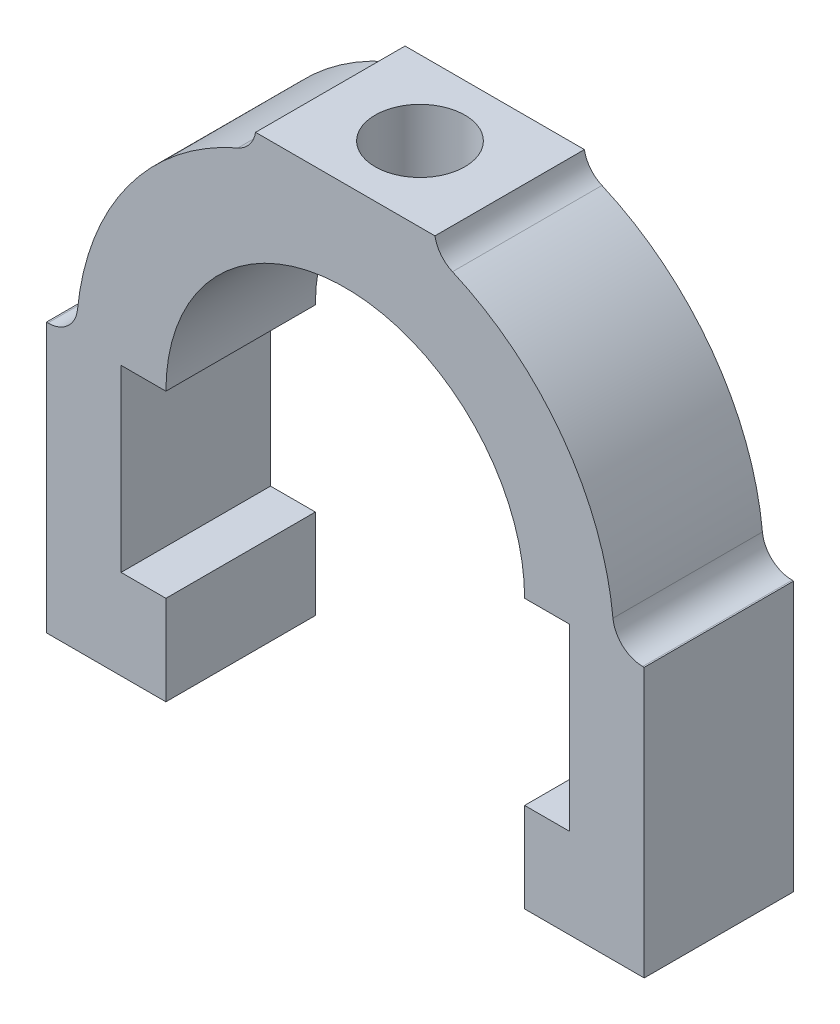
ISO-10303-21;
HEADER;
FILE_DESCRIPTION(('STEP AP214'),'2;1');
FILE_NAME('part.step','',(''),(''),'','','');
FILE_SCHEMA(('AUTOMOTIVE_DESIGN { 1 0 10303 214 1 1 1 1 }'));
ENDSEC;
DATA;
#1=APPLICATION_CONTEXT('core data for automotive mechanical design processes');
#2=APPLICATION_PROTOCOL_DEFINITION('international standard','automotive_design',2000,#1);
#3=PRODUCT_CONTEXT('',#1,'mechanical');
#4=PRODUCT('Part','Part','',(#3));
#5=PRODUCT_RELATED_PRODUCT_CATEGORY('part','',(#4));
#6=PRODUCT_DEFINITION_FORMATION('','',#4);
#7=PRODUCT_DEFINITION_CONTEXT('part definition',#1,'design');
#8=PRODUCT_DEFINITION('design','',#6,#7);
#9=PRODUCT_DEFINITION_SHAPE('','',#8);
#10=(LENGTH_UNIT() NAMED_UNIT(*) SI_UNIT(.MILLI.,.METRE.));
#11=(NAMED_UNIT(*) PLANE_ANGLE_UNIT() SI_UNIT($,.RADIAN.));
#12=(NAMED_UNIT(*) SI_UNIT($,.STERADIAN.) SOLID_ANGLE_UNIT());
#13=UNCERTAINTY_MEASURE_WITH_UNIT(LENGTH_MEASURE(1.E-05),#10,'distance_accuracy_value','');
#14=(GEOMETRIC_REPRESENTATION_CONTEXT(3) GLOBAL_UNCERTAINTY_ASSIGNED_CONTEXT((#13)) GLOBAL_UNIT_ASSIGNED_CONTEXT((#10,
#11,#12)) REPRESENTATION_CONTEXT('',''));
#15=CARTESIAN_POINT('',(0.,0.,0.));
#16=DIRECTION('',(0.,0.,1.));
#17=DIRECTION('',(1.,0.,0.));
#18=AXIS2_PLACEMENT_3D('',#15,#16,#17);
#19=CARTESIAN_POINT('',(0.,36.,-20.));
#20=DIRECTION('',(0.,0.,1.));
#21=DIRECTION('',(1.,0.,0.));
#22=AXIS2_PLACEMENT_3D('',#19,#20,#21);
#23=CYLINDRICAL_SURFACE('',#22,36.);
#24=CARTESIAN_POINT('',(0.,36.,-20.));
#25=DIRECTION('',(0.,0.,1.));
#26=DIRECTION('',(1.,0.,0.));
#27=AXIS2_PLACEMENT_3D('',#24,#25,#26);
#28=CIRCLE('',#27,36.);
#29=CARTESIAN_POINT('',(35.8195477358383,39.6,-20.));
#30=VERTEX_POINT('',#29);
#31=CARTESIAN_POINT('',(14.3465927559282,69.0178024146906,-20.));
#32=VERTEX_POINT('',#31);
#33=EDGE_CURVE('E302',#30,#32,#28,.T.);
#34=ORIENTED_EDGE('',*,*,#33,.T.);
#35=DIRECTION('',(0.,0.,1.));
#36=VECTOR('',#35,1.);
#37=CARTESIAN_POINT('',(14.3465927559282,69.0178024146906,-20.));
#38=LINE('',#37,#36);
#39=CARTESIAN_POINT('',(14.3465927559282,69.0178024146906,0.));
#40=VERTEX_POINT('',#39);
#41=EDGE_CURVE('E377',#32,#40,#38,.T.);
#42=ORIENTED_EDGE('',*,*,#41,.T.);
#43=CARTESIAN_POINT('',(0.,36.,0.));
#44=DIRECTION('',(0.,0.,1.));
#45=DIRECTION('',(1.,0.,0.));
#46=AXIS2_PLACEMENT_3D('',#43,#44,#45);
#47=CIRCLE('',#46,36.);
#48=CARTESIAN_POINT('',(35.8195477358383,39.6,0.));
#49=VERTEX_POINT('',#48);
#50=EDGE_CURVE('E330',#49,#40,#47,.T.);
#51=ORIENTED_EDGE('',*,*,#50,.F.);
#52=DIRECTION('',(0.,0.,1.));
#53=VECTOR('',#52,1.);
#54=CARTESIAN_POINT('',(35.8195477358383,39.6,-20.));
#55=LINE('',#54,#53);
#56=EDGE_CURVE('E361',#49,#30,#55,.F.);
#57=ORIENTED_EDGE('',*,*,#56,.T.);
#58=EDGE_LOOP('',(#34,#42,#51,#57));
#59=FACE_BOUND('',#58,.T.);
#60=ADVANCED_FACE('F58',(#59),#23,.T.);
#61=CARTESIAN_POINT('',(-14.3465927559282,69.0178024146906,0.));
#62=VERTEX_POINT('',#61);
#63=CARTESIAN_POINT('',(-35.8195477358383,39.6,0.));
#64=VERTEX_POINT('',#63);
#65=EDGE_CURVE('E327',#62,#64,#47,.T.);
#66=ORIENTED_EDGE('',*,*,#65,.F.);
#67=DIRECTION('',(0.,0.,1.));
#68=VECTOR('',#67,1.);
#69=CARTESIAN_POINT('',(-14.3465927559282,69.0178024146906,-20.));
#70=LINE('',#69,#68);
#71=CARTESIAN_POINT('',(-14.3465927559282,69.0178024146906,-20.));
#72=VERTEX_POINT('',#71);
#73=EDGE_CURVE('E84',#62,#72,#70,.F.);
#74=ORIENTED_EDGE('',*,*,#73,.T.);
#75=CARTESIAN_POINT('',(-35.8195477358383,39.6,-20.));
#76=VERTEX_POINT('',#75);
#77=EDGE_CURVE('E211',#72,#76,#28,.T.);
#78=ORIENTED_EDGE('',*,*,#77,.T.);
#79=DIRECTION('',(0.,0.,1.));
#80=VECTOR('',#79,1.);
#81=CARTESIAN_POINT('',(-35.8195477358383,39.6,-20.));
#82=LINE('',#81,#80);
#83=EDGE_CURVE('E367',#76,#64,#82,.T.);
#84=ORIENTED_EDGE('',*,*,#83,.T.);
#85=EDGE_LOOP('',(#66,#74,#78,#84));
#86=FACE_BOUND('',#85,.T.);
#87=ADVANCED_FACE('F462',(#86),#23,.T.);
#88=CARTESIAN_POINT('',(-24.,0.,-20.));
#89=DIRECTION('',(-1.,0.,0.));
#90=DIRECTION('',(0.,0.,1.));
#91=AXIS2_PLACEMENT_3D('',#88,#89,#90);
#92=PLANE('',#91);
#93=DIRECTION('',(0.,-1.,0.));
#94=VECTOR('',#93,1.);
#95=CARTESIAN_POINT('',(-24.,0.,-20.));
#96=LINE('',#95,#94);
#97=CARTESIAN_POINT('',(-24.,12.,-20.));
#98=VERTEX_POINT('',#97);
#99=CARTESIAN_POINT('',(-24.,0.,-20.));
#100=VERTEX_POINT('',#99);
#101=EDGE_CURVE('E314',#98,#100,#96,.T.);
#102=ORIENTED_EDGE('',*,*,#101,.F.);
#103=DIRECTION('',(0.,0.,1.));
#104=VECTOR('',#103,1.);
#105=CARTESIAN_POINT('',(-24.,12.,-178.));
#106=LINE('',#105,#104);
#107=CARTESIAN_POINT('',(-24.,12.,0.));
#108=VERTEX_POINT('',#107);
#109=EDGE_CURVE('E242',#98,#108,#106,.T.);
#110=ORIENTED_EDGE('',*,*,#109,.T.);
#111=DIRECTION('',(0.,-1.,0.));
#112=VECTOR('',#111,1.);
#113=CARTESIAN_POINT('',(-24.,0.,0.));
#114=LINE('',#113,#112);
#115=CARTESIAN_POINT('',(-24.,0.,0.));
#116=VERTEX_POINT('',#115);
#117=EDGE_CURVE('E294',#108,#116,#114,.T.);
#118=ORIENTED_EDGE('',*,*,#117,.T.);
#119=DIRECTION('',(0.,0.,1.));
#120=VECTOR('',#119,1.);
#121=CARTESIAN_POINT('',(-24.,0.,-20.));
#122=LINE('',#121,#120);
#123=EDGE_CURVE('E343',#100,#116,#122,.T.);
#124=ORIENTED_EDGE('',*,*,#123,.F.);
#125=EDGE_LOOP('',(#102,#110,#118,#124));
#126=FACE_BOUND('',#125,.T.);
#127=ADVANCED_FACE('F447',(#126),#92,.F.);
#128=CARTESIAN_POINT('',(0.,0.,-20.));
#129=DIRECTION('',(0.,-1.,0.));
#130=DIRECTION('',(0.,0.,-1.));
#131=AXIS2_PLACEMENT_3D('',#128,#129,#130);
#132=PLANE('',#131);
#133=DIRECTION('',(1.,0.,0.));
#134=VECTOR('',#133,1.);
#135=CARTESIAN_POINT('',(0.,0.,0.));
#136=LINE('',#135,#134);
#137=CARTESIAN_POINT('',(-40.,0.,0.));
#138=VERTEX_POINT('',#137);
#139=EDGE_CURVE('E340',#138,#116,#136,.T.);
#140=ORIENTED_EDGE('',*,*,#139,.F.);
#141=DIRECTION('',(0.,0.,1.));
#142=VECTOR('',#141,1.);
#143=CARTESIAN_POINT('',(-40.,0.,-20.));
#144=LINE('',#143,#142);
#145=CARTESIAN_POINT('',(-40.,0.,-20.));
#146=VERTEX_POINT('',#145);
#147=EDGE_CURVE('E349',#146,#138,#144,.T.);
#148=ORIENTED_EDGE('',*,*,#147,.F.);
#149=DIRECTION('',(1.,0.,0.));
#150=VECTOR('',#149,1.);
#151=CARTESIAN_POINT('',(0.,0.,-20.));
#152=LINE('',#151,#150);
#153=EDGE_CURVE('E315',#146,#100,#152,.T.);
#154=ORIENTED_EDGE('',*,*,#153,.T.);
#155=ORIENTED_EDGE('',*,*,#123,.T.);
#156=EDGE_LOOP('',(#140,#148,#154,#155));
#157=FACE_BOUND('',#156,.T.);
#158=ADVANCED_FACE('F446',(#157),#132,.T.);
#159=CARTESIAN_POINT('',(-40.,0.,-20.));
#160=DIRECTION('',(1.,0.,0.));
#161=DIRECTION('',(0.,0.,-1.));
#162=AXIS2_PLACEMENT_3D('',#159,#160,#161);
#163=PLANE('',#162);
#164=DIRECTION('',(0.,1.,0.));
#165=VECTOR('',#164,1.);
#166=CARTESIAN_POINT('',(-40.,0.,0.));
#167=LINE('',#166,#165);
#168=CARTESIAN_POINT('',(-40.,36.,0.));
#169=VERTEX_POINT('',#168);
#170=EDGE_CURVE('E332',#138,#169,#167,.T.);
#171=ORIENTED_EDGE('',*,*,#170,.T.);
#172=DIRECTION('',(0.,0.,1.));
#173=VECTOR('',#172,1.);
#174=CARTESIAN_POINT('',(-40.,36.,-20.));
#175=LINE('',#174,#173);
#176=CARTESIAN_POINT('',(-40.,36.,-20.));
#177=VERTEX_POINT('',#176);
#178=EDGE_CURVE('E350',#177,#169,#175,.T.);
#179=ORIENTED_EDGE('',*,*,#178,.F.);
#180=DIRECTION('',(0.,1.,0.));
#181=VECTOR('',#180,1.);
#182=CARTESIAN_POINT('',(-40.,0.,-20.));
#183=LINE('',#182,#181);
#184=EDGE_CURVE('E309',#146,#177,#183,.T.);
#185=ORIENTED_EDGE('',*,*,#184,.F.);
#186=ORIENTED_EDGE('',*,*,#147,.T.);
#187=EDGE_LOOP('',(#171,#179,#185,#186));
#188=FACE_BOUND('',#187,.T.);
#189=ADVANCED_FACE('F452',(#188),#163,.F.);
#190=CARTESIAN_POINT('',(0.,36.,-20.));
#191=DIRECTION('',(0.,-1.,0.));
#192=DIRECTION('',(0.,0.,-1.));
#193=AXIS2_PLACEMENT_3D('',#190,#191,#192);
#194=PLANE('',#193);
#195=DIRECTION('',(1.,0.,0.));
#196=VECTOR('',#195,1.);
#197=CARTESIAN_POINT('',(0.,36.,0.));
#198=LINE('',#197,#196);
#199=CARTESIAN_POINT('',(-39.7994974842648,36.,0.));
#200=VERTEX_POINT('',#199);
#201=EDGE_CURVE('E331',#169,#200,#198,.T.);
#202=ORIENTED_EDGE('',*,*,#201,.T.);
#203=DIRECTION('',(0.,0.,1.));
#204=VECTOR('',#203,1.);
#205=CARTESIAN_POINT('',(-39.7994974842648,36.,-20.));
#206=LINE('',#205,#204);
#207=CARTESIAN_POINT('',(-39.7994974842648,36.,-20.));
#208=VERTEX_POINT('',#207);
#209=EDGE_CURVE('E375',#200,#208,#206,.F.);
#210=ORIENTED_EDGE('',*,*,#209,.T.);
#211=DIRECTION('',(1.,0.,0.));
#212=VECTOR('',#211,1.);
#213=CARTESIAN_POINT('',(0.,36.,-20.));
#214=LINE('',#213,#212);
#215=EDGE_CURVE('E310',#177,#208,#214,.T.);
#216=ORIENTED_EDGE('',*,*,#215,.F.);
#217=ORIENTED_EDGE('',*,*,#178,.T.);
#218=EDGE_LOOP('',(#202,#210,#216,#217));
#219=FACE_BOUND('',#218,.T.);
#220=ADVANCED_FACE('F460',(#219),#194,.F.);
#221=CARTESIAN_POINT('',(0.,36.,-20.));
#222=DIRECTION('',(0.,1.,0.));
#223=DIRECTION('',(0.,0.,1.));
#224=AXIS2_PLACEMENT_3D('',#221,#222,#223);
#225=PLANE('',#224);
#226=DIRECTION('',(-1.,0.,0.));
#227=VECTOR('',#226,1.);
#228=CARTESIAN_POINT('',(0.,36.,-20.));
#229=LINE('',#228,#227);
#230=CARTESIAN_POINT('',(40.,36.,-20.));
#231=VERTEX_POINT('',#230);
#232=CARTESIAN_POINT('',(39.7994974842648,36.,-20.));
#233=VERTEX_POINT('',#232);
#234=EDGE_CURVE('E301',#231,#233,#229,.T.);
#235=ORIENTED_EDGE('',*,*,#234,.T.);
#236=DIRECTION('',(0.,0.,-1.));
#237=VECTOR('',#236,1.);
#238=CARTESIAN_POINT('',(39.7994974842648,36.,0.));
#239=LINE('',#238,#237);
#240=CARTESIAN_POINT('',(39.7994974842648,36.,0.));
#241=VERTEX_POINT('',#240);
#242=EDGE_CURVE('E345',#233,#241,#239,.F.);
#243=ORIENTED_EDGE('',*,*,#242,.T.);
#244=DIRECTION('',(-1.,0.,0.));
#245=VECTOR('',#244,1.);
#246=CARTESIAN_POINT('',(0.,36.,0.));
#247=LINE('',#246,#245);
#248=CARTESIAN_POINT('',(40.,36.,0.));
#249=VERTEX_POINT('',#248);
#250=EDGE_CURVE('E322',#249,#241,#247,.T.);
#251=ORIENTED_EDGE('',*,*,#250,.F.);
#252=DIRECTION('',(0.,0.,1.));
#253=VECTOR('',#252,1.);
#254=CARTESIAN_POINT('',(40.,36.,-20.));
#255=LINE('',#254,#253);
#256=EDGE_CURVE('E351',#231,#249,#255,.T.);
#257=ORIENTED_EDGE('',*,*,#256,.F.);
#258=EDGE_LOOP('',(#235,#243,#251,#257));
#259=FACE_BOUND('',#258,.T.);
#260=ADVANCED_FACE('F402',(#259),#225,.T.);
#261=CARTESIAN_POINT('',(40.,0.,-20.));
#262=DIRECTION('',(1.,0.,0.));
#263=DIRECTION('',(0.,0.,-1.));
#264=AXIS2_PLACEMENT_3D('',#261,#262,#263);
#265=PLANE('',#264);
#266=DIRECTION('',(0.,1.,0.));
#267=VECTOR('',#266,1.);
#268=CARTESIAN_POINT('',(40.,0.,0.));
#269=LINE('',#268,#267);
#270=CARTESIAN_POINT('',(40.,0.,0.));
#271=VERTEX_POINT('',#270);
#272=EDGE_CURVE('E321',#271,#249,#269,.T.);
#273=ORIENTED_EDGE('',*,*,#272,.F.);
#274=DIRECTION('',(0.,0.,1.));
#275=VECTOR('',#274,1.);
#276=CARTESIAN_POINT('',(40.,0.,-20.));
#277=LINE('',#276,#275);
#278=CARTESIAN_POINT('',(40.,0.,-20.));
#279=VERTEX_POINT('',#278);
#280=EDGE_CURVE('E353',#279,#271,#277,.T.);
#281=ORIENTED_EDGE('',*,*,#280,.F.);
#282=DIRECTION('',(0.,1.,0.));
#283=VECTOR('',#282,1.);
#284=CARTESIAN_POINT('',(40.,0.,-20.));
#285=LINE('',#284,#283);
#286=EDGE_CURVE('E296',#279,#231,#285,.T.);
#287=ORIENTED_EDGE('',*,*,#286,.T.);
#288=ORIENTED_EDGE('',*,*,#256,.T.);
#289=EDGE_LOOP('',(#273,#281,#287,#288));
#290=FACE_BOUND('',#289,.T.);
#291=ADVANCED_FACE('F403',(#290),#265,.T.);
#292=CARTESIAN_POINT('',(0.,0.,-20.));
#293=DIRECTION('',(0.,-1.,0.));
#294=DIRECTION('',(0.,0.,-1.));
#295=AXIS2_PLACEMENT_3D('',#292,#293,#294);
#296=PLANE('',#295);
#297=DIRECTION('',(1.,0.,0.));
#298=VECTOR('',#297,1.);
#299=CARTESIAN_POINT('',(0.,0.,0.));
#300=LINE('',#299,#298);
#301=CARTESIAN_POINT('',(24.,0.,0.));
#302=VERTEX_POINT('',#301);
#303=EDGE_CURVE('E316',#302,#271,#300,.T.);
#304=ORIENTED_EDGE('',*,*,#303,.F.);
#305=DIRECTION('',(0.,0.,1.));
#306=VECTOR('',#305,1.);
#307=CARTESIAN_POINT('',(24.,0.,-20.));
#308=LINE('',#307,#306);
#309=CARTESIAN_POINT('',(24.,0.,-20.));
#310=VERTEX_POINT('',#309);
#311=EDGE_CURVE('E358',#310,#302,#308,.T.);
#312=ORIENTED_EDGE('',*,*,#311,.F.);
#313=DIRECTION('',(1.,0.,0.));
#314=VECTOR('',#313,1.);
#315=CARTESIAN_POINT('',(0.,0.,-20.));
#316=LINE('',#315,#314);
#317=EDGE_CURVE('E295',#310,#279,#316,.T.);
#318=ORIENTED_EDGE('',*,*,#317,.T.);
#319=ORIENTED_EDGE('',*,*,#280,.T.);
#320=EDGE_LOOP('',(#304,#312,#318,#319));
#321=FACE_BOUND('',#320,.T.);
#322=ADVANCED_FACE('F413',(#321),#296,.T.);
#323=CARTESIAN_POINT('',(24.,0.,-20.));
#324=DIRECTION('',(-1.,0.,0.));
#325=DIRECTION('',(0.,0.,1.));
#326=AXIS2_PLACEMENT_3D('',#323,#324,#325);
#327=PLANE('',#326);
#328=DIRECTION('',(0.,0.,1.));
#329=VECTOR('',#328,1.);
#330=CARTESIAN_POINT('',(24.,12.,-178.));
#331=LINE('',#330,#329);
#332=CARTESIAN_POINT('',(24.,12.,-20.));
#333=VERTEX_POINT('',#332);
#334=CARTESIAN_POINT('',(24.,12.,0.));
#335=VERTEX_POINT('',#334);
#336=EDGE_CURVE('E248',#333,#335,#331,.T.);
#337=ORIENTED_EDGE('',*,*,#336,.F.);
#338=DIRECTION('',(0.,-1.,0.));
#339=VECTOR('',#338,1.);
#340=CARTESIAN_POINT('',(24.,0.,-20.));
#341=LINE('',#340,#339);
#342=EDGE_CURVE('E292',#333,#310,#341,.T.);
#343=ORIENTED_EDGE('',*,*,#342,.T.);
#344=ORIENTED_EDGE('',*,*,#311,.T.);
#345=DIRECTION('',(0.,-1.,0.));
#346=VECTOR('',#345,1.);
#347=CARTESIAN_POINT('',(24.,0.,0.));
#348=LINE('',#347,#346);
#349=EDGE_CURVE('E293',#335,#302,#348,.T.);
#350=ORIENTED_EDGE('',*,*,#349,.F.);
#351=EDGE_LOOP('',(#337,#343,#344,#350));
#352=FACE_BOUND('',#351,.T.);
#353=ADVANCED_FACE('F411',(#352),#327,.T.);
#354=CARTESIAN_POINT('',(0.,0.,-20.));
#355=DIRECTION('',(0.,0.,1.));
#356=DIRECTION('',(1.,0.,0.));
#357=AXIS2_PLACEMENT_3D('',#354,#355,#356);
#358=PLANE('',#357);
#359=DIRECTION('',(0.,1.,0.));
#360=VECTOR('',#359,1.);
#361=CARTESIAN_POINT('',(30.,0.,-20.));
#362=LINE('',#361,#360);
#363=CARTESIAN_POINT('',(30.,12.,-20.));
#364=VERTEX_POINT('',#363);
#365=CARTESIAN_POINT('',(30.,36.,-20.));
#366=VERTEX_POINT('',#365);
#367=EDGE_CURVE('E282',#364,#366,#362,.T.);
#368=ORIENTED_EDGE('',*,*,#367,.T.);
#369=DIRECTION('',(-1.,0.,0.));
#370=VECTOR('',#369,1.);
#371=CARTESIAN_POINT('',(0.,36.,-20.));
#372=LINE('',#371,#370);
#373=CARTESIAN_POINT('',(24.,36.,-20.));
#374=VERTEX_POINT('',#373);
#375=EDGE_CURVE('E272',#366,#374,#372,.T.);
#376=ORIENTED_EDGE('',*,*,#375,.T.);
#377=CARTESIAN_POINT('',(0.,36.,-20.));
#378=DIRECTION('',(0.,0.,1.));
#379=DIRECTION('',(1.,0.,0.));
#380=AXIS2_PLACEMENT_3D('',#377,#378,#379);
#381=CIRCLE('',#380,24.);
#382=CARTESIAN_POINT('',(-24.,36.,-20.));
#383=VERTEX_POINT('',#382);
#384=EDGE_CURVE('E290',#374,#383,#381,.T.);
#385=ORIENTED_EDGE('',*,*,#384,.T.);
#386=DIRECTION('',(-1.,0.,0.));
#387=VECTOR('',#386,1.);
#388=CARTESIAN_POINT('',(0.,36.,-20.));
#389=LINE('',#388,#387);
#390=CARTESIAN_POINT('',(-30.,36.,-20.));
#391=VERTEX_POINT('',#390);
#392=EDGE_CURVE('E255',#383,#391,#389,.T.);
#393=ORIENTED_EDGE('',*,*,#392,.T.);
#394=DIRECTION('',(0.,-1.,0.));
#395=VECTOR('',#394,1.);
#396=CARTESIAN_POINT('',(-30.,0.,-20.));
#397=LINE('',#396,#395);
#398=CARTESIAN_POINT('',(-30.,12.,-20.));
#399=VERTEX_POINT('',#398);
#400=EDGE_CURVE('E274',#391,#399,#397,.T.);
#401=ORIENTED_EDGE('',*,*,#400,.T.);
#402=DIRECTION('',(1.,0.,0.));
#403=VECTOR('',#402,1.);
#404=CARTESIAN_POINT('',(0.,12.,-20.));
#405=LINE('',#404,#403);
#406=EDGE_CURVE('E276',#399,#98,#405,.T.);
#407=ORIENTED_EDGE('',*,*,#406,.T.);
#408=ORIENTED_EDGE('',*,*,#101,.T.);
#409=ORIENTED_EDGE('',*,*,#153,.F.);
#410=ORIENTED_EDGE('',*,*,#184,.T.);
#411=ORIENTED_EDGE('',*,*,#215,.T.);
#412=CARTESIAN_POINT('',(-39.7994974842648,40.,-20.));
#413=DIRECTION('',(0.,0.,1.));
#414=DIRECTION('',(1.,0.,0.));
#415=AXIS2_PLACEMENT_3D('',#412,#413,#414);
#416=CIRCLE('',#415,4.);
#417=EDGE_CURVE('E376',#208,#76,#416,.T.);
#418=ORIENTED_EDGE('',*,*,#417,.T.);
#419=ORIENTED_EDGE('',*,*,#77,.F.);
#420=CARTESIAN_POINT('',(-15.940658617698,72.686447127434,-20.));
#421=DIRECTION('',(0.,0.,1.));
#422=DIRECTION('',(1.,0.,0.));
#423=AXIS2_PLACEMENT_3D('',#420,#421,#422);
#424=CIRCLE('',#423,4.);
#425=CARTESIAN_POINT('',(-12.,72.,-20.));
#426=VERTEX_POINT('',#425);
#427=EDGE_CURVE('E12',#72,#426,#424,.T.);
#428=ORIENTED_EDGE('',*,*,#427,.T.);
#429=DIRECTION('',(1.,0.,0.));
#430=VECTOR('',#429,1.);
#431=CARTESIAN_POINT('',(0.,72.,-20.));
#432=LINE('',#431,#430);
#433=CARTESIAN_POINT('',(12.,72.,-20.));
#434=VERTEX_POINT('',#433);
#435=EDGE_CURVE('E209',#426,#434,#432,.T.);
#436=ORIENTED_EDGE('',*,*,#435,.T.);
#437=CARTESIAN_POINT('',(15.940658617698,72.686447127434,-20.));
#438=DIRECTION('',(0.,0.,1.));
#439=DIRECTION('',(1.,0.,0.));
#440=AXIS2_PLACEMENT_3D('',#437,#438,#439);
#441=CIRCLE('',#440,4.);
#442=EDGE_CURVE('E384',#434,#32,#441,.T.);
#443=ORIENTED_EDGE('',*,*,#442,.T.);
#444=ORIENTED_EDGE('',*,*,#33,.F.);
#445=CARTESIAN_POINT('',(39.7994974842648,40.,-20.));
#446=DIRECTION('',(0.,0.,1.));
#447=DIRECTION('',(1.,0.,0.));
#448=AXIS2_PLACEMENT_3D('',#445,#446,#447);
#449=CIRCLE('',#448,4.);
#450=EDGE_CURVE('E370',#30,#233,#449,.T.);
#451=ORIENTED_EDGE('',*,*,#450,.T.);
#452=ORIENTED_EDGE('',*,*,#234,.F.);
#453=ORIENTED_EDGE('',*,*,#286,.F.);
#454=ORIENTED_EDGE('',*,*,#317,.F.);
#455=ORIENTED_EDGE('',*,*,#342,.F.);
#456=DIRECTION('',(1.,0.,0.));
#457=VECTOR('',#456,1.);
#458=CARTESIAN_POINT('',(0.,12.,-20.));
#459=LINE('',#458,#457);
#460=EDGE_CURVE('E277',#333,#364,#459,.T.);
#461=ORIENTED_EDGE('',*,*,#460,.T.);
#462=EDGE_LOOP('',(#368,#376,#385,#393,#401,#407,#408,#409,#410,#411,#418,#419,#428,#436,#443,
#444,#451,#452,#453,#454,#455,#461));
#463=FACE_BOUND('',#462,.T.);
#464=ADVANCED_FACE('F206',(#463),#358,.F.);
#465=CARTESIAN_POINT('',(0.,0.,0.));
#466=DIRECTION('',(0.,0.,1.));
#467=DIRECTION('',(1.,0.,0.));
#468=AXIS2_PLACEMENT_3D('',#465,#466,#467);
#469=PLANE('',#468);
#470=DIRECTION('',(-1.,0.,0.));
#471=VECTOR('',#470,1.);
#472=CARTESIAN_POINT('',(30.,36.,0.));
#473=LINE('',#472,#471);
#474=CARTESIAN_POINT('',(30.,36.,0.));
#475=VERTEX_POINT('',#474);
#476=CARTESIAN_POINT('',(24.,36.,0.));
#477=VERTEX_POINT('',#476);
#478=EDGE_CURVE('E250',#475,#477,#473,.T.);
#479=ORIENTED_EDGE('',*,*,#478,.F.);
#480=DIRECTION('',(0.,1.,0.));
#481=VECTOR('',#480,1.);
#482=CARTESIAN_POINT('',(30.,12.,0.));
#483=LINE('',#482,#481);
#484=CARTESIAN_POINT('',(30.,12.,0.));
#485=VERTEX_POINT('',#484);
#486=EDGE_CURVE('E243',#485,#475,#483,.T.);
#487=ORIENTED_EDGE('',*,*,#486,.F.);
#488=DIRECTION('',(1.,0.,0.));
#489=VECTOR('',#488,1.);
#490=CARTESIAN_POINT('',(24.,12.,0.));
#491=LINE('',#490,#489);
#492=EDGE_CURVE('E239',#335,#485,#491,.T.);
#493=ORIENTED_EDGE('',*,*,#492,.F.);
#494=ORIENTED_EDGE('',*,*,#349,.T.);
#495=ORIENTED_EDGE('',*,*,#303,.T.);
#496=ORIENTED_EDGE('',*,*,#272,.T.);
#497=ORIENTED_EDGE('',*,*,#250,.T.);
#498=CARTESIAN_POINT('',(39.7994974842648,40.,0.));
#499=DIRECTION('',(0.,0.,1.));
#500=DIRECTION('',(1.,0.,0.));
#501=AXIS2_PLACEMENT_3D('',#498,#499,#500);
#502=CIRCLE('',#501,4.);
#503=EDGE_CURVE('E362',#241,#49,#502,.F.);
#504=ORIENTED_EDGE('',*,*,#503,.T.);
#505=ORIENTED_EDGE('',*,*,#50,.T.);
#506=CARTESIAN_POINT('',(15.940658617698,72.686447127434,0.));
#507=DIRECTION('',(0.,0.,1.));
#508=DIRECTION('',(1.,0.,0.));
#509=AXIS2_PLACEMENT_3D('',#506,#507,#508);
#510=CIRCLE('',#509,4.);
#511=CARTESIAN_POINT('',(12.,72.,0.));
#512=VERTEX_POINT('',#511);
#513=EDGE_CURVE('E382',#40,#512,#510,.F.);
#514=ORIENTED_EDGE('',*,*,#513,.T.);
#515=DIRECTION('',(1.,0.,0.));
#516=VECTOR('',#515,1.);
#517=CARTESIAN_POINT('',(0.,72.,0.));
#518=LINE('',#517,#516);
#519=CARTESIAN_POINT('',(-12.,72.,0.));
#520=VERTEX_POINT('',#519);
#521=EDGE_CURVE('E225',#520,#512,#518,.T.);
#522=ORIENTED_EDGE('',*,*,#521,.F.);
#523=CARTESIAN_POINT('',(-15.940658617698,72.686447127434,0.));
#524=DIRECTION('',(0.,0.,1.));
#525=DIRECTION('',(1.,0.,0.));
#526=AXIS2_PLACEMENT_3D('',#523,#524,#525);
#527=CIRCLE('',#526,4.);
#528=EDGE_CURVE('E67',#520,#62,#527,.F.);
#529=ORIENTED_EDGE('',*,*,#528,.T.);
#530=ORIENTED_EDGE('',*,*,#65,.T.);
#531=CARTESIAN_POINT('',(-39.7994974842648,40.,0.));
#532=DIRECTION('',(0.,0.,1.));
#533=DIRECTION('',(1.,0.,0.));
#534=AXIS2_PLACEMENT_3D('',#531,#532,#533);
#535=CIRCLE('',#534,4.);
#536=EDGE_CURVE('E372',#64,#200,#535,.F.);
#537=ORIENTED_EDGE('',*,*,#536,.T.);
#538=ORIENTED_EDGE('',*,*,#201,.F.);
#539=ORIENTED_EDGE('',*,*,#170,.F.);
#540=ORIENTED_EDGE('',*,*,#139,.T.);
#541=ORIENTED_EDGE('',*,*,#117,.F.);
#542=DIRECTION('',(1.,0.,0.));
#543=VECTOR('',#542,1.);
#544=CARTESIAN_POINT('',(-24.,12.,0.));
#545=LINE('',#544,#543);
#546=CARTESIAN_POINT('',(-30.,12.,0.));
#547=VERTEX_POINT('',#546);
#548=EDGE_CURVE('E263',#547,#108,#545,.T.);
#549=ORIENTED_EDGE('',*,*,#548,.F.);
#550=DIRECTION('',(0.,-1.,0.));
#551=VECTOR('',#550,1.);
#552=CARTESIAN_POINT('',(-30.,12.,0.));
#553=LINE('',#552,#551);
#554=CARTESIAN_POINT('',(-30.,36.,0.));
#555=VERTEX_POINT('',#554);
#556=EDGE_CURVE('E260',#555,#547,#553,.T.);
#557=ORIENTED_EDGE('',*,*,#556,.F.);
#558=DIRECTION('',(-1.,0.,0.));
#559=VECTOR('',#558,1.);
#560=CARTESIAN_POINT('',(-30.,36.,0.));
#561=LINE('',#560,#559);
#562=CARTESIAN_POINT('',(-24.,36.,0.));
#563=VERTEX_POINT('',#562);
#564=EDGE_CURVE('E237',#563,#555,#561,.T.);
#565=ORIENTED_EDGE('',*,*,#564,.F.);
#566=CARTESIAN_POINT('',(0.,36.,0.));
#567=DIRECTION('',(0.,0.,1.));
#568=DIRECTION('',(1.,0.,0.));
#569=AXIS2_PLACEMENT_3D('',#566,#567,#568);
#570=CIRCLE('',#569,24.);
#571=EDGE_CURVE('E281',#477,#563,#570,.T.);
#572=ORIENTED_EDGE('',*,*,#571,.F.);
#573=EDGE_LOOP('',(#479,#487,#493,#494,#495,#496,#497,#504,#505,#514,#522,#529,#530,#537,#538,
#539,#540,#541,#549,#557,#565,#572));
#574=FACE_BOUND('',#573,.T.);
#575=ADVANCED_FACE('F395',(#574),#469,.T.);
#576=CARTESIAN_POINT('',(39.7994974842648,40.,-20.));
#577=DIRECTION('',(0.,0.,1.));
#578=DIRECTION('',(1.,0.,0.));
#579=AXIS2_PLACEMENT_3D('',#576,#577,#578);
#580=CYLINDRICAL_SURFACE('',#579,4.);
#581=ORIENTED_EDGE('',*,*,#450,.F.);
#582=ORIENTED_EDGE('',*,*,#56,.F.);
#583=ORIENTED_EDGE('',*,*,#503,.F.);
#584=ORIENTED_EDGE('',*,*,#242,.F.);
#585=EDGE_LOOP('',(#581,#582,#583,#584));
#586=FACE_BOUND('',#585,.T.);
#587=ADVANCED_FACE('F399',(#586),#580,.F.);
#588=CARTESIAN_POINT('',(-39.7994974842648,40.,-20.));
#589=DIRECTION('',(0.,0.,1.));
#590=DIRECTION('',(1.,0.,0.));
#591=AXIS2_PLACEMENT_3D('',#588,#589,#590);
#592=CYLINDRICAL_SURFACE('',#591,4.);
#593=ORIENTED_EDGE('',*,*,#417,.F.);
#594=ORIENTED_EDGE('',*,*,#209,.F.);
#595=ORIENTED_EDGE('',*,*,#536,.F.);
#596=ORIENTED_EDGE('',*,*,#83,.F.);
#597=EDGE_LOOP('',(#593,#594,#595,#596));
#598=FACE_BOUND('',#597,.T.);
#599=ADVANCED_FACE('F465',(#598),#592,.F.);
#600=CARTESIAN_POINT('',(0.,36.,-31.));
#601=DIRECTION('',(0.,0.,1.));
#602=DIRECTION('',(1.,0.,0.));
#603=AXIS2_PLACEMENT_3D('',#600,#601,#602);
#604=CYLINDRICAL_SURFACE('',#603,24.);
#605=CARTESIAN_POINT('',(0.,60.,-4.));
#606=CARTESIAN_POINT('',(0.165805387403802,60.0000029962766,-3.99999505102641));
#607=CARTESIAN_POINT('',(0.331556618095783,59.9982792337243,-4.00687387489243));
#608=CARTESIAN_POINT('',(0.661898341499742,59.9914389070726,-4.03431986201637));
#609=CARTESIAN_POINT('',(0.826488699612241,59.9863219558732,-4.05488858704015));
#610=CARTESIAN_POINT('',(1.15331468289425,59.9728312747808,-4.10955571939549));
#611=CARTESIAN_POINT('',(1.31554956136034,59.964456534561,-4.14365832400845));
#612=CARTESIAN_POINT('',(1.63652999353389,59.9446785682942,-4.22512392789649));
#613=CARTESIAN_POINT('',(1.7952742379173,59.9332742261501,-4.27249181441513));
#614=CARTESIAN_POINT('',(2.10785890827135,59.9077704080524,-4.38001719827038));
#615=CARTESIAN_POINT('',(2.26170674963502,59.8936752583917,-4.44015418258226));
#616=CARTESIAN_POINT('',(2.56378623821258,59.8631527081916,-4.57282541021577));
#617=CARTESIAN_POINT('',(2.71201578712804,59.8467244469549,-4.64536423066248));
#618=CARTESIAN_POINT('',(3.00177661033544,59.8119848981805,-4.80226274512907));
#619=CARTESIAN_POINT('',(3.1433102969363,59.7936742964516,-4.88661813795178));
#620=CARTESIAN_POINT('',(3.41888526654491,59.7556431475739,-5.06661176459039));
#621=CARTESIAN_POINT('',(3.5529237053449,59.7359220715781,-5.1622542392442));
#622=CARTESIAN_POINT('',(3.81496434602383,59.6952304700178,-5.36598591724915));
#623=CARTESIAN_POINT('',(3.94281308913214,59.674243775966,-5.47426931255561));
#624=CARTESIAN_POINT('',(4.18902736841679,59.6319204183454,-5.70115303311099));
#625=CARTESIAN_POINT('',(4.30738936846955,59.6105836278175,-5.8197571713109));
#626=CARTESIAN_POINT('',(4.53377489524013,59.568159620478,-6.06643888329868));
#627=CARTESIAN_POINT('',(4.64180103185486,59.5470723418473,-6.19451405100954));
#628=CARTESIAN_POINT('',(4.84686316299839,59.5057198367545,-6.45938141653677));
#629=CARTESIAN_POINT('',(4.94389508557169,59.4854549166434,-6.59617681496597));
#630=CARTESIAN_POINT('',(5.12757579334232,59.4460427828086,-6.87960061394558));
#631=CARTESIAN_POINT('',(5.21405329073272,59.4269160793509,-7.02634297896338));
#632=CARTESIAN_POINT('',(5.37434099239073,59.3906650895731,-7.32689631114159));
#633=CARTESIAN_POINT('',(5.4481464054103,59.3735415614194,-7.48070992415988));
#634=CARTESIAN_POINT('',(5.5824381696205,59.3418328254504,-7.79422880998301));
#635=CARTESIAN_POINT('',(5.64293112700069,59.3272463593972,-7.95393111442795));
#636=CARTESIAN_POINT('',(5.75016256060697,59.301043510543,-8.27812298906709));
#637=CARTESIAN_POINT('',(5.79689611131117,59.2894281915327,-8.4426142504887));
#638=CARTESIAN_POINT('',(5.91415157316671,59.2600431044562,-8.93482169258661));
#639=CARTESIAN_POINT('',(5.96458986092324,59.2470332112981,-9.26798361707615));
#640=CARTESIAN_POINT('',(5.99795848349603,59.23842608856,-9.77014845136033));
#641=CARTESIAN_POINT('',(6.00202663613951,59.2373766993858,-9.93800547716951));
#642=CARTESIAN_POINT('',(5.99610970800768,59.2389046091482,-10.2734756491558));
#643=CARTESIAN_POINT('',(5.98612448822742,59.2414819439575,-10.4410887929042));
#644=CARTESIAN_POINT('',(5.93594713474591,59.2543754061852,-10.9334757617709));
#645=CARTESIAN_POINT('',(5.87607363848321,59.2697164452628,-11.2563322349699));
#646=CARTESIAN_POINT('',(5.70489646981085,59.3122664593645,-11.8870944582585));
#647=CARTESIAN_POINT('',(5.59358913348967,59.3394762798586,-12.1949991415238));
#648=CARTESIAN_POINT('',(5.32155798729425,59.4030050803747,-12.7909383990231));
#649=CARTESIAN_POINT('',(5.16034668919655,59.4394132393811,-13.0787410216454));
#650=CARTESIAN_POINT('',(4.79342508379137,59.5171882932266,-13.623678505182));
#651=CARTESIAN_POINT('',(4.58770698972655,59.5585560552156,-13.8808079874003));
#652=CARTESIAN_POINT('',(4.13065370439076,59.6430352608536,-14.3648134392708));
#653=CARTESIAN_POINT('',(3.8781850342093,59.6861627896442,-14.5906176860606));
#654=CARTESIAN_POINT('',(3.33844766846889,59.7682386126258,-14.9968852440488));
#655=CARTESIAN_POINT('',(3.05117791031428,59.8071867791381,-15.1773471702746));
#656=CARTESIAN_POINT('',(2.44846355524484,59.8767092866155,-15.4882022714257));
#657=CARTESIAN_POINT('',(2.13292557335861,59.9072544059235,-15.6184213427058));
#658=CARTESIAN_POINT('',(1.48350403204752,59.9563166788424,-15.8236692411467));
#659=CARTESIAN_POINT('',(1.14962399502517,59.9748361331613,-15.8987086254555));
#660=CARTESIAN_POINT('',(0.482159883096527,59.9974199712544,-15.9898302624469));
#661=CARTESIAN_POINT('',(0.148786885522348,60.0018421411353,-16.0073721225199));
#662=CARTESIAN_POINT('',(-0.516131504775042,59.9967521917739,-15.987003973561));
#663=CARTESIAN_POINT('',(-0.847677059317268,59.987241326857,-15.94909895615));
#664=CARTESIAN_POINT('',(-1.4944570546744,59.9555832478693,-15.8201164380113));
#665=CARTESIAN_POINT('',(-1.80986040015949,59.9336253776701,-15.7298352125968));
#666=CARTESIAN_POINT('',(-2.42102924553322,59.8795482551267,-15.4995713973546));
#667=CARTESIAN_POINT('',(-2.71679275860286,59.8474279766146,-15.3595837881582));
#668=CARTESIAN_POINT('',(-3.28609225023473,59.775732355911,-15.0310564967388));
#669=CARTESIAN_POINT('',(-3.55914068563651,59.7360348408855,-14.8416993592124));
#670=CARTESIAN_POINT('',(-4.07010753646662,59.6537802212633,-14.4208365553548));
#671=CARTESIAN_POINT('',(-4.30801987625634,59.6112226239559,-14.1893236149746));
#672=CARTESIAN_POINT('',(-4.74795813275242,59.5267588379479,-13.6840067323829));
#673=CARTESIAN_POINT('',(-4.94895984477464,59.4848942795269,-13.4093042078171));
#674=CARTESIAN_POINT('',(-5.30205866107054,59.4077130231476,-12.8290144447531));
#675=CARTESIAN_POINT('',(-5.45415793615243,59.3723960345683,-12.5234285779765));
#676=CARTESIAN_POINT('',(-5.6416087071287,59.3275859445682,-12.0496398809846));
#677=CARTESIAN_POINT('',(-5.69722158138527,59.3140336618751,-11.8895567217037));
#678=CARTESIAN_POINT('',(-5.79475769208554,59.2899834650234,-11.5650651703049));
#679=CARTESIAN_POINT('',(-5.83668611505733,59.2794843938355,-11.4006584424464));
#680=CARTESIAN_POINT('',(-5.9064899745362,59.2618715740422,-11.0687170513407));
#681=CARTESIAN_POINT('',(-5.93436517338602,59.2547578826878,-10.901182335245));
#682=CARTESIAN_POINT('',(-5.97582085063046,59.2441396190328,-10.5642421336349));
#683=CARTESIAN_POINT('',(-5.98940200008078,59.2406348773048,-10.3948367363199));
#684=CARTESIAN_POINT('',(-6.00196347285349,59.2373938489065,-10.060331055056));
#685=CARTESIAN_POINT('',(-6.0013522054121,59.2375521518778,-9.89524696865287));
#686=CARTESIAN_POINT('',(-5.98653576306369,59.2413736324535,-9.56573349984315));
#687=CARTESIAN_POINT('',(-5.97233089751311,59.2450367302975,-9.401304102623));
#688=CARTESIAN_POINT('',(-5.93044575509701,59.2557579721328,-9.07425896558782));
#689=CARTESIAN_POINT('',(-5.90276341290372,59.2628166364686,-8.91164350765425));
#690=CARTESIAN_POINT('',(-5.83416667908453,59.2801148571724,-8.58946233314158));
#691=CARTESIAN_POINT('',(-5.79325695086328,59.2903532924404,-8.42989556269428));
#692=CARTESIAN_POINT('',(-5.69880203716712,59.3136441790929,-8.11574761367387));
#693=CARTESIAN_POINT('',(-5.64532943643257,59.3266804293978,-7.96114338738971));
#694=CARTESIAN_POINT('',(-5.52605852883571,59.3552228194459,-7.65706577641293));
#695=CARTESIAN_POINT('',(-5.46026449802037,59.3707281020539,-7.50759063294574));
#696=CARTESIAN_POINT('',(-5.31678835542035,59.4037855982137,-7.21461325501314));
#697=CARTESIAN_POINT('',(-5.23910089912543,59.4213387311534,-7.07111374285786));
#698=CARTESIAN_POINT('',(-5.07243073970643,59.4579990976357,-6.79110854339098));
#699=CARTESIAN_POINT('',(-4.98345174049215,59.4771058208267,-6.65460058319193));
#700=CARTESIAN_POINT('',(-4.7922729032838,59.5168854335111,-6.38585732091633));
#701=CARTESIAN_POINT('',(-4.68978556121475,59.5375863850894,-6.25383061677941));
#702=CARTESIAN_POINT('',(-4.4742434518464,59.579507882839,-5.99887487156699));
#703=CARTESIAN_POINT('',(-4.36119228671727,59.6007282500856,-5.87594275475177));
#704=CARTESIAN_POINT('',(-4.12516419546942,59.6431258862839,-5.63985111466564));
#705=CARTESIAN_POINT('',(-4.0021814457299,59.6643031223737,-5.52669740687929));
#706=CARTESIAN_POINT('',(-3.74719176501411,59.7060168559164,-5.31103132209644));
#707=CARTESIAN_POINT('',(-3.61518813420472,59.7265535837286,-5.2085150877252));
#708=CARTESIAN_POINT('',(-3.34044186706076,59.7668061369628,-5.0129768060556));
#709=CARTESIAN_POINT('',(-3.19754553860501,59.7864996932668,-4.92016593894123));
#710=CARTESIAN_POINT('',(-2.90425652857033,59.824087485808,-4.74697329866601));
#711=CARTESIAN_POINT('',(-2.75386663022821,59.8419823827553,-4.66658695566752));
#712=CARTESIAN_POINT('',(-2.44663692885418,59.8754647710401,-4.51885051284106));
#713=CARTESIAN_POINT('',(-2.28979994155171,59.8910532562916,-4.45149479378778));
#714=CARTESIAN_POINT('',(-1.97079001830644,59.9194829588902,-4.3303336445071));
#715=CARTESIAN_POINT('',(-1.80861789148404,59.9323245906257,-4.27652617018404));
#716=CARTESIAN_POINT('',(-1.3777763047293,59.9619049568243,-4.15376714609566));
#717=CARTESIAN_POINT('',(-1.1055914726577,59.9761014751911,-4.09620462215925));
#718=CARTESIAN_POINT('',(-0.55555350244454,59.9951461360495,-4.01932663186095));
#719=CARTESIAN_POINT('',(-0.277700792219541,59.9999949816564,-4.00000828883734));
#720=CARTESIAN_POINT('',(0.,60.,-4.));
#721=B_SPLINE_CURVE_WITH_KNOTS('',3,(#605,#606,#607,#608,#609,#610,#611,#612,#613,#614,#615,
#616,#617,#618,#619,#620,#621,#622,#623,#624,#625,#626,#627,#628,#629,#630,#631,#632,#633,#634,
#635,#636,#637,#638,#639,#640,#641,#642,#643,#644,#645,#646,#647,#648,#649,#650,#651,#652,#653,
#654,#655,#656,#657,#658,#659,#660,#661,#662,#663,#664,#665,#666,#667,#668,#669,#670,#671,#672,
#673,#674,#675,#676,#677,#678,#679,#680,#681,#682,#683,#684,#685,#686,#687,#688,#689,#690,#691,
#692,#693,#694,#695,#696,#697,#698,#699,#700,#701,#702,#703,#704,#705,#706,#707,#708,#709,#710,
#711,#712,#713,#714,#715,#716,#717,#718,#719,#720),.UNSPECIFIED.,.T.,.F.,(4,2,2,2,2,2,2,2,2,2,2,
2,2,2,2,2,2,2,2,2,2,2,2,2,2,2,2,2,2,2,2,2,2,2,2,2,2,2,2,2,2,2,2,2,2,2,2,2,2,2,2,2,2,2,2,2,2,4),
(0.,0.497171453608337,0.994399635056343,1.49178214324908,1.98934814054333,2.48612078574438,
2.98307717135303,3.47985313409878,3.97681634579052,4.48278784834555,4.98894707988207,
5.49497816255321,6.00119605682159,6.51476681838441,7.02853133276356,7.54204031819885,
8.0557329040678,9.06140626133586,9.56463055957973,10.0678598353591,11.0489981911534,
12.0302064495334,13.021319425847,14.0126059443383,15.0321583496526,16.0517418932217,
17.0748274712564,18.0977172584376,19.0944306688629,20.0910543554016,21.0729092914533,
22.0548634037835,23.0542418135059,24.0537928312126,25.0778786790709,26.1019190608722,
26.6114255778037,27.1207387624019,27.6300605598219,28.1393584452954,28.6340191333343,
29.1286685643954,29.6233938208458,30.1179448483897,30.6097058740945,31.10129655354,
31.593108789452,32.0847601135969,32.5894192432003,33.0939069121446,33.5986925778495,
34.1032945530712,34.6172488082311,35.1310135748031,35.6445562931573,36.1580214841036,
36.9907766489356,37.8234691729712),.UNSPECIFIED.);
#722=CARTESIAN_POINT('',(0.,60.,-4.));
#723=VERTEX_POINT('',#722);
#724=EDGE_CURVE('E222',#723,#723,#721,.T.);
#725=ORIENTED_EDGE('',*,*,#724,.T.);
#726=EDGE_LOOP('',(#725));
#727=FACE_BOUND('',#726,.T.);
#728=DIRECTION('',(0.,0.,1.));
#729=VECTOR('',#728,1.);
#730=CARTESIAN_POINT('',(24.,36.,-20.));
#731=LINE('',#730,#729);
#732=EDGE_CURVE('E320',#374,#477,#731,.T.);
#733=ORIENTED_EDGE('',*,*,#732,.T.);
#734=ORIENTED_EDGE('',*,*,#571,.T.);
#735=DIRECTION('',(0.,0.,1.));
#736=VECTOR('',#735,1.);
#737=CARTESIAN_POINT('',(-24.,36.,-20.));
#738=LINE('',#737,#736);
#739=EDGE_CURVE('E344',#383,#563,#738,.T.);
#740=ORIENTED_EDGE('',*,*,#739,.F.);
#741=ORIENTED_EDGE('',*,*,#384,.F.);
#742=EDGE_LOOP('',(#733,#734,#740,#741));
#743=FACE_BOUND('',#742,.T.);
#744=ADVANCED_FACE('F429',(#727,#743),#604,.F.);
#745=CARTESIAN_POINT('',(-24.,12.,-178.));
#746=DIRECTION('',(0.,-1.,0.));
#747=DIRECTION('',(0.,0.,-1.));
#748=AXIS2_PLACEMENT_3D('',#745,#746,#747);
#749=PLANE('',#748);
#750=DIRECTION('',(0.,0.,1.));
#751=VECTOR('',#750,1.);
#752=CARTESIAN_POINT('',(-30.,12.,-178.));
#753=LINE('',#752,#751);
#754=EDGE_CURVE('E269',#399,#547,#753,.T.);
#755=ORIENTED_EDGE('',*,*,#754,.T.);
#756=ORIENTED_EDGE('',*,*,#548,.T.);
#757=ORIENTED_EDGE('',*,*,#109,.F.);
#758=ORIENTED_EDGE('',*,*,#406,.F.);
#759=EDGE_LOOP('',(#755,#756,#757,#758));
#760=FACE_BOUND('',#759,.T.);
#761=ADVANCED_FACE('F508',(#760),#749,.F.);
#762=CARTESIAN_POINT('',(-30.,12.,-178.));
#763=DIRECTION('',(-1.,0.,0.));
#764=DIRECTION('',(0.,0.,1.));
#765=AXIS2_PLACEMENT_3D('',#762,#763,#764);
#766=PLANE('',#765);
#767=DIRECTION('',(0.,0.,1.));
#768=VECTOR('',#767,1.);
#769=CARTESIAN_POINT('',(-30.,36.,-178.));
#770=LINE('',#769,#768);
#771=EDGE_CURVE('E262',#391,#555,#770,.T.);
#772=ORIENTED_EDGE('',*,*,#771,.T.);
#773=ORIENTED_EDGE('',*,*,#556,.T.);
#774=ORIENTED_EDGE('',*,*,#754,.F.);
#775=ORIENTED_EDGE('',*,*,#400,.F.);
#776=EDGE_LOOP('',(#772,#773,#774,#775));
#777=FACE_BOUND('',#776,.T.);
#778=ADVANCED_FACE('F439',(#777),#766,.F.);
#779=CARTESIAN_POINT('',(-30.,36.,-178.));
#780=DIRECTION('',(0.,1.,0.));
#781=DIRECTION('',(0.,0.,1.));
#782=AXIS2_PLACEMENT_3D('',#779,#780,#781);
#783=PLANE('',#782);
#784=ORIENTED_EDGE('',*,*,#739,.T.);
#785=ORIENTED_EDGE('',*,*,#564,.T.);
#786=ORIENTED_EDGE('',*,*,#771,.F.);
#787=ORIENTED_EDGE('',*,*,#392,.F.);
#788=EDGE_LOOP('',(#784,#785,#786,#787));
#789=FACE_BOUND('',#788,.T.);
#790=ADVANCED_FACE('F433',(#789),#783,.F.);
#791=CARTESIAN_POINT('',(30.,12.,-178.));
#792=DIRECTION('',(1.,0.,0.));
#793=DIRECTION('',(0.,0.,-1.));
#794=AXIS2_PLACEMENT_3D('',#791,#792,#793);
#795=PLANE('',#794);
#796=DIRECTION('',(0.,0.,1.));
#797=VECTOR('',#796,1.);
#798=CARTESIAN_POINT('',(30.,12.,-178.));
#799=LINE('',#798,#797);
#800=EDGE_CURVE('E254',#364,#485,#799,.T.);
#801=ORIENTED_EDGE('',*,*,#800,.T.);
#802=ORIENTED_EDGE('',*,*,#486,.T.);
#803=DIRECTION('',(0.,0.,1.));
#804=VECTOR('',#803,1.);
#805=CARTESIAN_POINT('',(30.,36.,-178.));
#806=LINE('',#805,#804);
#807=EDGE_CURVE('E249',#366,#475,#806,.T.);
#808=ORIENTED_EDGE('',*,*,#807,.F.);
#809=ORIENTED_EDGE('',*,*,#367,.F.);
#810=EDGE_LOOP('',(#801,#802,#808,#809));
#811=FACE_BOUND('',#810,.T.);
#812=ADVANCED_FACE('F422',(#811),#795,.F.);
#813=CARTESIAN_POINT('',(24.,12.,-178.));
#814=DIRECTION('',(0.,-1.,0.));
#815=DIRECTION('',(0.,0.,-1.));
#816=AXIS2_PLACEMENT_3D('',#813,#814,#815);
#817=PLANE('',#816);
#818=ORIENTED_EDGE('',*,*,#336,.T.);
#819=ORIENTED_EDGE('',*,*,#492,.T.);
#820=ORIENTED_EDGE('',*,*,#800,.F.);
#821=ORIENTED_EDGE('',*,*,#460,.F.);
#822=EDGE_LOOP('',(#818,#819,#820,#821));
#823=FACE_BOUND('',#822,.T.);
#824=ADVANCED_FACE('F420',(#823),#817,.F.);
#825=CARTESIAN_POINT('',(30.,36.,-178.));
#826=DIRECTION('',(0.,1.,0.));
#827=DIRECTION('',(0.,0.,1.));
#828=AXIS2_PLACEMENT_3D('',#825,#826,#827);
#829=PLANE('',#828);
#830=ORIENTED_EDGE('',*,*,#807,.T.);
#831=ORIENTED_EDGE('',*,*,#478,.T.);
#832=ORIENTED_EDGE('',*,*,#732,.F.);
#833=ORIENTED_EDGE('',*,*,#375,.F.);
#834=EDGE_LOOP('',(#830,#831,#832,#833));
#835=FACE_BOUND('',#834,.T.);
#836=ADVANCED_FACE('F424',(#835),#829,.F.);
#837=CARTESIAN_POINT('',(0.,72.,-20.));
#838=DIRECTION('',(0.,-1.,0.));
#839=DIRECTION('',(0.,0.,-1.));
#840=AXIS2_PLACEMENT_3D('',#837,#838,#839);
#841=PLANE('',#840);
#842=CARTESIAN_POINT('',(0.,72.,-10.));
#843=DIRECTION('',(0.,1.,0.));
#844=DIRECTION('',(0.,0.,1.));
#845=AXIS2_PLACEMENT_3D('',#842,#843,#844);
#846=CIRCLE('',#845,6.);
#847=CARTESIAN_POINT('',(0.,72.,-4.));
#848=VERTEX_POINT('',#847);
#849=EDGE_CURVE('E230',#848,#848,#846,.T.);
#850=ORIENTED_EDGE('',*,*,#849,.F.);
#851=EDGE_LOOP('',(#850));
#852=FACE_BOUND('',#851,.T.);
#853=ORIENTED_EDGE('',*,*,#521,.T.);
#854=DIRECTION('',(0.,0.,1.));
#855=VECTOR('',#854,1.);
#856=CARTESIAN_POINT('',(12.,72.,-20.));
#857=LINE('',#856,#855);
#858=EDGE_CURVE('E224',#434,#512,#857,.T.);
#859=ORIENTED_EDGE('',*,*,#858,.F.);
#860=ORIENTED_EDGE('',*,*,#435,.F.);
#861=DIRECTION('',(0.,0.,1.));
#862=VECTOR('',#861,1.);
#863=CARTESIAN_POINT('',(-12.,72.,-20.));
#864=LINE('',#863,#862);
#865=EDGE_CURVE('E220',#426,#520,#864,.T.);
#866=ORIENTED_EDGE('',*,*,#865,.T.);
#867=EDGE_LOOP('',(#853,#859,#860,#866));
#868=FACE_BOUND('',#867,.T.);
#869=ADVANCED_FACE('F217',(#852,#868),#841,.F.);
#870=CARTESIAN_POINT('',(15.940658617698,72.686447127434,-20.));
#871=DIRECTION('',(0.,0.,-1.));
#872=DIRECTION('',(-1.,0.,0.));
#873=AXIS2_PLACEMENT_3D('',#870,#871,#872);
#874=CYLINDRICAL_SURFACE('',#873,4.);
#875=ORIENTED_EDGE('',*,*,#442,.F.);
#876=ORIENTED_EDGE('',*,*,#858,.T.);
#877=ORIENTED_EDGE('',*,*,#513,.F.);
#878=ORIENTED_EDGE('',*,*,#41,.F.);
#879=EDGE_LOOP('',(#875,#876,#877,#878));
#880=FACE_BOUND('',#879,.T.);
#881=ADVANCED_FACE('F394',(#880),#874,.F.);
#882=CARTESIAN_POINT('',(-15.940658617698,72.686447127434,-20.));
#883=DIRECTION('',(0.,0.,-1.));
#884=DIRECTION('',(-1.,0.,0.));
#885=AXIS2_PLACEMENT_3D('',#882,#883,#884);
#886=CYLINDRICAL_SURFACE('',#885,4.);
#887=ORIENTED_EDGE('',*,*,#427,.F.);
#888=ORIENTED_EDGE('',*,*,#73,.F.);
#889=ORIENTED_EDGE('',*,*,#528,.F.);
#890=ORIENTED_EDGE('',*,*,#865,.F.);
#891=EDGE_LOOP('',(#887,#888,#889,#890));
#892=FACE_BOUND('',#891,.T.);
#893=ADVANCED_FACE('F61',(#892),#886,.F.);
#894=CARTESIAN_POINT('',(0.,52.,-10.));
#895=DIRECTION('',(0.,1.,0.));
#896=DIRECTION('',(0.,0.,1.));
#897=AXIS2_PLACEMENT_3D('',#894,#895,#896);
#898=CYLINDRICAL_SURFACE('',#897,6.);
#899=ORIENTED_EDGE('',*,*,#849,.T.);
#900=EDGE_LOOP('',(#899));
#901=FACE_BOUND('',#900,.T.);
#902=ORIENTED_EDGE('',*,*,#724,.F.);
#903=EDGE_LOOP('',(#902));
#904=FACE_BOUND('',#903,.T.);
#905=ADVANCED_FACE('F495',(#901,#904),#898,.F.);
#906=CLOSED_SHELL('',(#60,#87,#127,#158,#189,#220,#260,#291,#322,#353,#464,#575,#587,#599,#744,
#761,#778,#790,#812,#824,#836,#869,#881,#893,#905));
#907=MANIFOLD_SOLID_BREP('B2',#906);
#908=ADVANCED_BREP_SHAPE_REPRESENTATION('',(#18,#907),#14);
#909=SHAPE_DEFINITION_REPRESENTATION(#9,#908);
ENDSEC;
END-ISO-10303-21;
